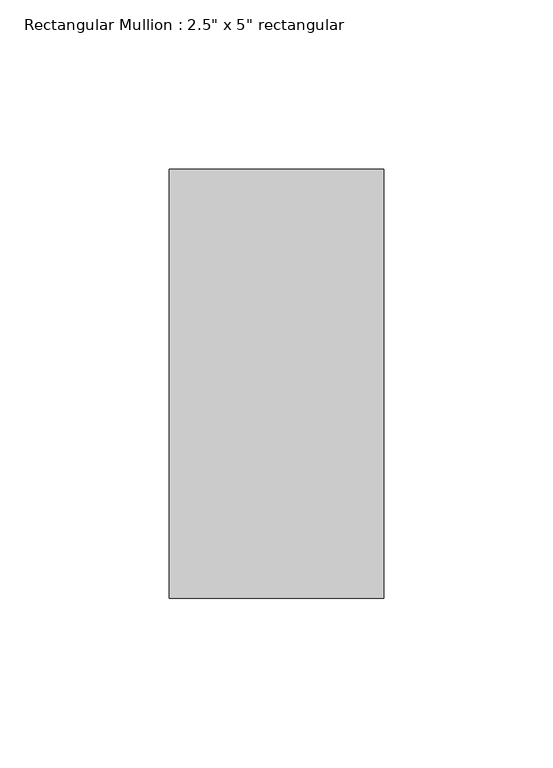
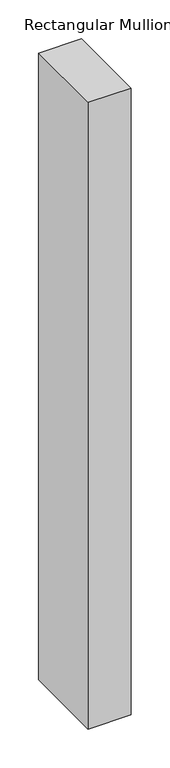
"""IFC4 building model written with IfcOpenShell, lengths in millimetres: member geometry."""

from ifc_helpers import new_model, si_unit, frame, origin, place, context, project, spatial, polyline, outline, extrude, source, transform, mapped, element, save


def member_7f5bebbe(model_context):
    return source(origin(), model_context, "Body", "SweptSolid", [
        extrude(outline(polyline([(0.0, 63.5), (0.0, -63.5), (-63.5, -63.5), (-63.5, 63.5), (0.0, 63.5)])), frame((0.0, 0.0, -983.0943516), z_axis=(0.0, 0.0, 1.0), x_axis=(1.0, 0.0, 0.0)), (0.0, 0.0, 1.0), 983.0943516),
    ])


if __name__ == "__main__":
    model = new_model("IFC4")
    model_context = context("Model", 3, world=origin())
    ifc_project = project(units=[si_unit("LENGTHUNIT", "METRE", prefix="MILLI")], contexts=[model_context])
    site = spatial("IfcSite", under=ifc_project)
    building = spatial("IfcBuilding", under=site)
    placement = place(None, origin())
    member_shape = member_7f5bebbe(model_context)
    element("IfcMember", 1, ObjectType="Rectangular Mullion : 2.5\" x 5\" rectangular", at=placement, inside=building, context=model_context, shape_type="MappedRepresentation", body=[
        mapped(member_shape, transform((0.0, 0.0, 0.0), x_axis=(1.0, 0.0, 0.0), y_axis=(0.0, 1.0, 0.0), z_axis=(0.0, 0.0, 1.0))),
    ])
    save(model, "model.ifc")

# Revit data of these elements
# Type "Rectangular Mullion : 2.5\" x 5\" rectangular"
#   built-in parameter 1007304 = 0.416667 (stored number, unit not read)
#   built-in parameter 1007301 = 0.104167 (stored number, unit not read)
#   built-in parameter 1007300 = 0.104167 (stored number, unit not read)
# Element 1 (IfcMember, "Rectangular Mullion : 2.5\" x 5\" rectangular")
#   Materials on its faces: "Aluminum"
# Materials
#   "Aluminum": class "Metal", colour RGB 247 247 247, transparency 0, Description = "Aluminum 6061", Cost = 0
